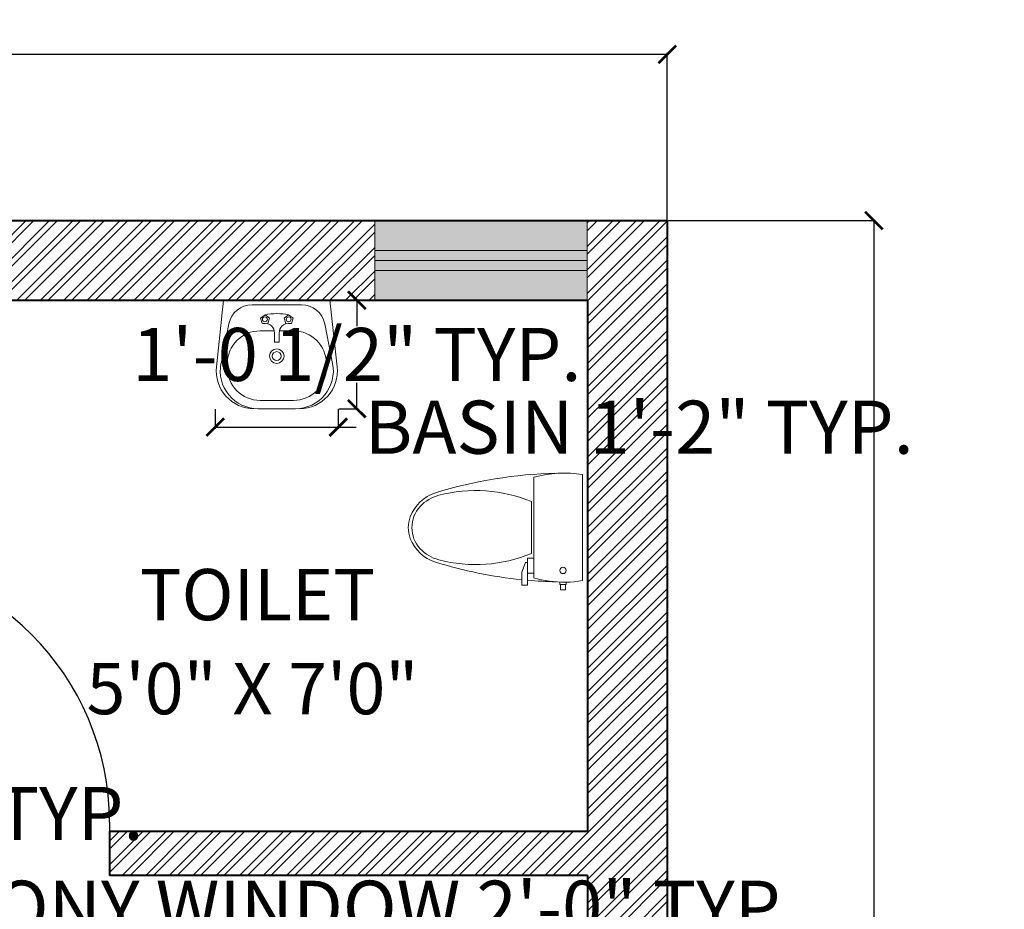
# Model space of a CAD drawing. Units: inches. Extents: x 528 to 2520, y -151 to 1354.
# Tile 27 of 41: x 1350 to 1461, y 1239 to 1340. Entities that reach past the tile are written whole.
import ezdxf

# ---------------------------------------------------------------- set-up
doc = ezdxf.new("R2010")
doc.units = ezdxf.units.IN
doc.header["$MEASUREMENT"] = 0
for name, color, linetype, lineweight in [('A-ANNO-DIMS', 2, 'Continuous', 18), ('A-AREA-IDEN', 7, 'Continuous', 18), ('A-Door', 150, 'Continuous', 25), ('A-FLOR-FIXT', 9, 'Continuous', 18), ('A-WALL-PATT', 6, 'Continuous', 13), ('walls', 7, 'Continuous', 40), ('WINDOWS', 2, 'Continuous', 20)]:
    doc.layers.add(name, color=color, linetype=linetype, lineweight=lineweight)
doc.layers.add('A-GLAZ-PATT', color=152, linetype='Continuous', lineweight=13, true_color=0x2776bb)
doc.styles.get("Standard").update_dxf_attribs({"font": 'arial.ttf'})
doc.dimstyles.get("Standard").update_dxf_attribs({"dimtxt": 6, "dimasz": 2, "dimexe": 0.18, "dimexo": 0.0625, "dimgap": 0.09, "dimtad": 0, "dimtih": 1, "dimtoh": 1, "dimdec": 1, "dimzin": 0, "dimdsep": 46, "dimlunit": 3, "dimtxsty": 'Standard', "dimblk": 'ARCHTICK', "dimcen": 0.09, "dimadec": 0, "dimazin": 0, "dimtfac": 1, "dimtdec": 1, "dimtofl": 0, "dimtmove": 0, "dimatfit": 3, "dimfxl": 1, "dimtolj": 1, "dimtzin": 0, "dimarcsym": 0})

# ---------------------------------------------------------------- blocks, each defined once
blk = doc.blocks.new('toilet-7')
at = {"color": 0, "linetype": 'ByBlock'}
for p, q in [((0.2097, -0.02), (-0.2097, -0.02)), ((0.2151, -0.0677), (0.2097, -0.02)), ((0.2151, -0.1171), (0.2151, -0.0677)), ((-0.2457, -0.0874), (-0.2457, -0.1068)), ((-0.2457, -0.0874), (-0.2257, -0.0874)), ((-0.2457, -0.1068), (-0.2257, -0.1068)), ((-0.2257, -0.0846), (-0.2257, -0.1096)), ((-0.2257, -0.0846), (-0.2157, -0.0846)), ((-0.2257, -0.1096), (-0.2154, -0.1096)), ((0.2099, -0.164), (0.2151, -0.1171)), ((0.1991, -0.2124), (0.2099, -0.164)), ((0.1991, -0.2124), (-0.1991, -0.2124)), ((-0.1803, -0.2374), (-0.1803, -0.2124)), ((-0.1213, -0.2374), (-0.1213, -0.2124)), ((-0.1023, -0.2212), (0.1023, -0.2212)), ((-0.1213, -0.2374), (-0.2278, -0.2374)), ((-0.2278, -0.2374), (-0.2278, -0.2599)), ((-0.1759, -0.2599), (-0.2278, -0.2599)), ((-0.1759, -0.2599), (-0.1379, -0.2451)), ((-0.1379, -0.2451), (-0.1379, -0.2374))]:
    blk.add_line(p, q, dxfattribs=at)
blk.add_circle((-0.1696, -0.0971), 0.0125, dxfattribs=at)
for centre, radius, start, end in [((0.2244, -0.0924), 0.4402, 170.5377, 187.7399), ((1.517, -0.087), 1.7318, 181.2224, 184.9822), ((0.2244, -0.0924), 0.4402, 187.7399, 195.822), ((-1.517, -0.087), 1.7318, 342.7523, 358.7776), ((0.4258, -0.4413), 0.5721, 157.3737, 194.7786), ((-0.4258, -0.4413), 0.5721, 345.2214, 22.6263), ((1.517, -0.087), 1.7318, 185.7323, 197.2477), ((0.0116, -0.5544), 0.1554, 197.2477, 249.5476), ((0.0221, -0.5478), 0.1546, 194.7786, 226.8543), ((-0.0116, -0.5544), 0.1554, 290.4524, 342.7523), ((-0.0221, -0.5478), 0.1546, 313.1457, 345.2214), ((0, -0.5713), 0.1223, 226.8543, 313.1457), ((0, -0.5854), 0.1223, 249.5476, 290.4524)]:
    blk.add_arc(centre, radius, start, end, dxfattribs=at)
blk = doc.blocks.new('_ArchTick')
at = {"color": 0, "linetype": 'ByBlock', "const_width": 0.15}
blk.add_lwpolyline([(-0.5, -0.5), (0.5, 0.5)], dxfattribs=at)
blk = doc.blocks.new('*D26')
at = {"layer": 'A-ANNO-DIMS', "color": 0, "lineweight": -2, "transparency": 16777216}
for p, q in [((1422.95, 1317.1), (1446.41, 1317.1)), ((1446.23, 1317.1), (1446.23, 1069.76)), ((1446.23, 816.1), (1446.23, 1063.45)), ((1422.95, 816.1), (1446.41, 816.1))]:
    blk.add_line(p, q, dxfattribs=at)
at = {"layer": 'Defpoints', "color": 0, "transparency": 16777216}
for p in [(1422.88, 1317.1), (1422.88, 816.1), (1446.23, 816.1)]:
    blk.add_point(p, dxfattribs=at)
at = {"layer": 'A-ANNO-DIMS', "color": 0, "lineweight": -2, "transparency": 16777216, "xscale": 2, "yscale": 2, "zscale": 2}
for p, rotation in [((1446.23, 1317.1), 90), ((1446.23, 816.1), 270)]:
    blk.add_blockref('_ArchTick', p, dxfattribs=dict(at, rotation=rotation))
at = {"layer": 'A-ANNO-DIMS', "color": 0, "transparency": 16777216, "insert": (1446.23, 1066.6), "char_height": 6, "attachment_point": 5}
blk.add_mtext('\\A1;41\'-9.0"', dxfattribs=at)
blk = doc.blocks.new('*D27')
at = {"layer": 'A-ANNO-DIMS', "color": 0, "lineweight": -2, "transparency": 16777216}
for p, q in [((1123.88, 1317.17), (1123.88, 1336.05)), ((1123.88, 1335.87), (1257.11, 1335.87)), ((1422.88, 1335.87), (1289.66, 1335.87)), ((1422.88, 1317.17), (1422.88, 1336.05))]:
    blk.add_line(p, q, dxfattribs=at)
at = {"layer": 'Defpoints', "color": 0, "transparency": 16777216}
for p in [(1422.88, 1335.87), (1123.88, 1317.1), (1422.88, 1317.1)]:
    blk.add_point(p, dxfattribs=at)
at = {"layer": 'A-ANNO-DIMS', "color": 0, "lineweight": -2, "transparency": 16777216, "xscale": 2, "yscale": 2, "zscale": 2, "rotation": 180}
blk.add_blockref('_ArchTick', (1123.88, 1335.87), dxfattribs=at)
at = {"layer": 'A-ANNO-DIMS', "color": 0, "lineweight": -2, "transparency": 16777216, "xscale": 2, "yscale": 2, "zscale": 2}
blk.add_blockref('_ArchTick', (1422.88, 1335.87), dxfattribs=at)
at = {"layer": 'A-ANNO-DIMS', "color": 0, "transparency": 16777216, "insert": (1273.38, 1335.87), "char_height": 6, "attachment_point": 5}
blk.add_mtext('\\A1;24\'-11.0"', dxfattribs=at)
blk = doc.blocks.new('BASIN-WITH-TAP')
for p, q in [((0.84, 12.27), (0.02, 4.73)), ((12.84, 12.27), (0.84, 12.27)), ((12.84, 12.27), (13.66, 4.73)), ((9.64, 11.73), (4.05, 11.73)), ((5, 10.24), (5.51, 10.61)), ((5.2, 9.64), (5, 10.24)), ((5.24, 10.1), (5.2, 10.1)), ((5.51, 10.61), (6.02, 10.24)), ((6.02, 10.24), (5.82, 9.64)), ((8.18, 10.61), (7.67, 10.24)), ((7.67, 10.24), (7.86, 9.64)), ((8.68, 10.24), (8.18, 10.61)), ((8.44, 10.1), (8.49, 10.1)), ((8.49, 9.64), (8.68, 10.24)), ((1.43, 9.58), (0.55, 5.09)), ((5.24, 9.64), (5.51, 9.64)), ((8.49, 9.64), (8.18, 9.64)), ((12.26, 9.58), (13.14, 5.09)), ((4.98, 8.8), (6.58, 8.8)), ((6.58, 8.31), (6.58, 8.58)), ((6.58, 7.51), (6.58, 8.31)), ((8.71, 8.8), (7.11, 8.8)), ((7.11, 8.31), (7.11, 8.58)), ((7.11, 7.51), (7.11, 8.31)), ((6.58, 7.51), (7.11, 7.51)), ((1.24, 4.67), (1.24, 5.07)), ((12.44, 4.67), (12.44, 5.07)), ((4.73, 0), (8.96, 0)), ((6.84, 0.93), (4.98, 0.93)), ((6.84, 0.93), (8.71, 0.93))]:
    blk.add_line(p, q)
for centre, radius in [((5.5, 10.1), 0.277), ((8.19, 10.1), 0.277), ((6.84, 5.94), 0.821), ((6.84, 5.94), 0.507)]:
    blk.add_circle(centre, radius)
for centre, radius, start, end in [((4.05, 9.07), 2.67, 90, 168.8773), ((9.64, 9.07), 2.67, 11.1227, 90), ((6.84, 4.01), 6.73, 78.5788, 101.4212), ((5.51, 8.58), 1.07, 0, 90), ((8.18, 8.58), 1.07, 90, 180), ((4.98, 5.07), 3.73, 90, 180), ((8.71, 5.07), 3.73, 0, 90), ((4.27, 4.27), 4.27, 173.7966, 270), ((4.73, 4.27), 4.27, 168.8773, 270), ((4.98, 4.67), 3.73, 180, 270), ((8.71, 4.67), 3.73, 270, 0), ((8.96, 4.27), 4.27, 270, 11.1227), ((9.42, 4.27), 4.27, 270, 6.2034)]:
    blk.add_arc(centre, radius, start, end)
blk = doc.blocks.new('DOOR-SWING-30')
for p, q in [((0, 6), (0, 0)), ((30, 6), (30, 0))]:
    blk.add_line(p, q)
blk.add_lwpolyline([(0, 6), (0, 36), (1.75, 36), (1.75, 6)], close=True)
blk.add_arc((0, 6), 30, 0, 90)
blk = doc.blocks.new('WINDOW-24x9-PLAN')
for p, q in [((0, 5.63), (24, 5.63)), ((0, 4.5), (24, 4.5)), ((0, 3.37), (24, 3.37))]:
    blk.add_line(p, q)
blk.add_lwpolyline([(0, 9), (24, 9), (24, 0), (0, 0)], close=True)
blk = doc.blocks.new('*D52')
at = {"layer": 'A-ANNO-DIMS', "color": 0, "lineweight": -2, "transparency": 16777216}
for p, q in [((1371.83, 1295.77), (1371.83, 1293.57)), ((1385.73, 1295.77), (1385.73, 1293.57)), ((1371.83, 1293.75), (1385.73, 1293.75)), ((1385.73, 1293.75), (1387.73, 1293.75))]:
    blk.add_line(p, q, dxfattribs=at)
at = {"layer": 'Defpoints', "color": 0, "transparency": 16777216}
for p in [(1371.83, 1295.84), (1385.73, 1295.84), (1385.73, 1293.75)]:
    blk.add_point(p, dxfattribs=at)
at = {"layer": 'A-ANNO-DIMS', "color": 0, "lineweight": -2, "transparency": 16777216, "xscale": 2, "yscale": 2, "zscale": 2, "rotation": 180}
blk.add_blockref('_ArchTick', (1371.83, 1293.75), dxfattribs=at)
at = {"layer": 'A-ANNO-DIMS', "color": 0, "lineweight": -2, "transparency": 16777216, "xscale": 2, "yscale": 2, "zscale": 2}
blk.add_blockref('_ArchTick', (1385.73, 1293.75), dxfattribs=at)
at = {"layer": 'A-ANNO-DIMS', "color": 0, "transparency": 16777216, "insert": (1419.72, 1293.75), "char_height": 6, "attachment_point": 5}
blk.add_mtext('\\A1;BASIN 1\'-2" TYP.', dxfattribs=at)
blk = doc.blocks.new('*D53')
at = {"layer": 'A-ANNO-DIMS', "color": 0, "lineweight": -2, "transparency": 16777216}
for p, q in [((1385.8, 1308.1), (1388, 1308.1)), ((1387.82, 1308.1), (1387.82, 1305.16)), ((1387.82, 1295.84), (1387.82, 1298.78)), ((1385.8, 1295.84), (1388, 1295.84))]:
    blk.add_line(p, q, dxfattribs=at)
at = {"layer": 'Defpoints', "color": 0, "transparency": 16777216}
for p in [(1385.73, 1308.1), (1387.82, 1308.1), (1385.73, 1295.84)]:
    blk.add_point(p, dxfattribs=at)
at = {"layer": 'A-ANNO-DIMS', "color": 0, "lineweight": -2, "transparency": 16777216, "xscale": 2, "yscale": 2, "zscale": 2}
for p, rotation in [((1387.82, 1308.1), 90), ((1387.82, 1295.84), 270)]:
    blk.add_blockref('_ArchTick', p, dxfattribs=dict(at, rotation=rotation))
at = {"layer": 'A-ANNO-DIMS', "color": 0, "transparency": 16777216, "insert": (1387.82, 1301.97), "char_height": 6, "attachment_point": 5}
blk.add_mtext('\\A1;1\'-0 1/2" TYP.', dxfattribs=at)
blk = doc.blocks.new('*D86')
at = {"layer": 'A-ANNO-DIMS', "color": 0, "lineweight": -2, "transparency": 16777216}
for p, q in [((1297.45, 1243.04), (1297.45, 1239.32)), ((1321.45, 1243.04), (1321.45, 1239.32)), ((1297.45, 1239.5), (1321.45, 1239.5)), ((1321.45, 1239.5), (1323.45, 1239.5))]:
    blk.add_line(p, q, dxfattribs=at)
at = {"layer": 'Defpoints', "color": 0, "transparency": 16777216}
for p in [(1297.45, 1243.1), (1321.45, 1243.1), (1321.45, 1239.5)]:
    blk.add_point(p, dxfattribs=at)
at = {"layer": 'A-ANNO-DIMS', "color": 0, "lineweight": -2, "transparency": 16777216, "xscale": 2, "yscale": 2, "zscale": 2, "rotation": 180}
blk.add_blockref('_ArchTick', (1297.45, 1239.5), dxfattribs=at)
at = {"layer": 'A-ANNO-DIMS', "color": 0, "lineweight": -2, "transparency": 16777216, "xscale": 2, "yscale": 2, "zscale": 2}
blk.add_blockref('_ArchTick', (1321.45, 1239.5), dxfattribs=at)
at = {"layer": 'A-ANNO-DIMS', "color": 0, "transparency": 16777216, "insert": (1382.44, 1239.5), "char_height": 6, "attachment_point": 5}
blk.add_mtext('\\A1;BALCONY WINDOW 2\'-0" TYP.', dxfattribs=at)
blk = doc.blocks.new('*D87')
at = {"layer": 'A-ANNO-DIMS', "color": 0, "lineweight": -2, "transparency": 16777216}
for p, q in [((1325.05, 1248.1), (1325.05, 1250.1)), ((1325.05, 1250.1), (1327.05, 1250.1)), ((1321.51, 1248.1), (1325.23, 1248.1)), ((1325.05, 1243.1), (1325.05, 1248.1)), ((1321.51, 1243.1), (1325.23, 1243.1))]:
    blk.add_line(p, q, dxfattribs=at)
at = {"layer": 'Defpoints', "color": 0, "transparency": 16777216}
for p in [(1321.45, 1248.1), (1325.05, 1248.1), (1321.45, 1243.1)]:
    blk.add_point(p, dxfattribs=at)
at = {"layer": 'A-ANNO-DIMS', "color": 0, "lineweight": -2, "transparency": 16777216, "xscale": 2, "yscale": 2, "zscale": 2}
for p, rotation in [((1325.05, 1248.1), 90), ((1325.05, 1243.1), 270)]:
    blk.add_blockref('_ArchTick', p, dxfattribs=dict(at, rotation=rotation))
at = {"layer": 'A-ANNO-DIMS', "color": 0, "transparency": 16777216, "insert": (1345.43, 1250.1), "char_height": 6, "attachment_point": 5}
blk.add_mtext('\\A1;0\'-5" TYP.', dxfattribs=at)

msp = doc.modelspace()

# ---------------------------------------------------------------- hatches: boundary and pattern name
at = {"layer": 'A-GLAZ-PATT'}
h = msp.add_hatch(color=256, dxfattribs=at)
h.dxf.hatch_style = 1
h.paths.add_polyline_path([(1413.84, 1313.73), (1389.84, 1313.73), (1389.84, 1312.6), (1413.84, 1312.6)])
h.paths.add_polyline_path([(1413.84, 1312.6), (1389.84, 1312.6), (1389.84, 1311.47), (1413.84, 1311.47)])
h.paths.add_polyline_path([(1413.84, 1317.1), (1389.84, 1317.1), (1389.84, 1313.73), (1413.84, 1313.73)])
h.paths.add_polyline_path([(1413.84, 1311.47), (1389.84, 1311.47), (1389.84, 1308.1), (1413.84, 1308.1)])
at = {"layer": 'A-WALL-PATT'}
h = msp.add_hatch(dxfattribs=at)
h.set_pattern_fill('ANSI32', color=256, scale=5)
h.set_pattern_definition([(45, (537.1868, 0), (-1.3258252, 1.3258252), []), (45, (538.0707, 0), (-1.3258252, 1.3258252), [])])
h.paths.add_polyline_path([(1132.88, 1163.86), (1123.88, 1163.86), (1123.88, 969.1), (1135.43, 969.1), (1140.43, 969.1), (1140.43, 974.1), (1132.88, 974.1), (1132.88, 1082.1), (1228.88, 1082.1), (1228.88, 1087.1), (1228.88, 1106.1), (1234.88, 1106.1), (1234.88, 1111.1), (1223.88, 1111.1), (1223.88, 1087.1), (1132.88, 1087.1)])
h.paths.add_polyline_path([(1225.89, 974.1), (1188.43, 974.1), (1188.43, 969.1), (1225.89, 969.1)])
h.paths.add_polyline_path([(1422.88, 1171.37), (1413.88, 1171.37), (1413.88, 1111.1), (1323.88, 1111.1), (1323.88, 1106.1), (1413.88, 1106.1), (1413.88, 974.1), (1323.88, 974.1), (1323.88, 969.1), (1413.88, 969.1), (1413.88, 825.1), (1371.88, 825.1), (1371.88, 816.1), (1422.88, 816.1)])
h.paths.add_polyline_path([(1422.88, 1317.1), (1413.84, 1317.1), (1413.84, 1308.1), (1413.88, 1308.1), (1413.88, 1248.1), (1359.88, 1248.1), (1359.88, 1243.1), (1413.88, 1243.1), (1413.88, 1219.37), (1422.88, 1219.37)])
h.paths.add_polyline_path([(1389.84, 1317.1), (1324.88, 1317.1), (1324.88, 1248.1), (1321.45, 1248.1), (1321.45, 1243.1), (1329.88, 1243.1), (1329.88, 1249.1), (1329.88, 1308.1), (1389.84, 1308.1)])
h.paths.add_polyline_path([(1221.88, 1317.1), (1156.88, 1317.1), (1156.88, 1308.1), (1216.88, 1308.1), (1216.88, 1248.1), (1216.88, 1243.1), (1221.88, 1243.1), (1221.88, 1248.25)])
h.paths.add_polyline_path([(1132.88, 1308.1), (1132.88, 1317.1), (1123.88, 1317.1), (1123.88, 1211.86), (1132.88, 1211.86), (1132.88, 1243.1), (1186.88, 1243.1), (1186.88, 1248.1), (1132.88, 1248.1)])
h.paths.add_polyline_path([(1281.88, 969.1), (1281.88, 974.1), (1261.89, 974.1), (1261.89, 969.1), (1276.88, 969.1), (1276.88, 874.29), (1281.88, 874.29)])
h.paths.add_polyline_path([(1276.88, 969.1), (1264.88, 969.1), (1264.88, 965.12), (1267.92, 965.12), (1267.92, 961.68), (1271.62, 961.68), (1271.62, 957.24), (1276.88, 957.24)], flags=17)
h.paths.add_polyline_path([(1323.88, 825.1), (1281.88, 825.1), (1281.88, 832.29), (1276.88, 832.29), (1276.88, 816.1), (1323.88, 816.1)])

# ---------------------------------------------------------------- linework, layer by layer
at = {"layer": 'walls'}
for p, q in [((1324.88, 1317.1), (1422.88, 1317.1)), ((1422.88, 1317.1), (1422.88, 816.1)), ((1329.88, 1308.1), (1413.88, 1308.1)), ((1413.88, 1308.1), (1413.88, 1248.1)), ((1359.88, 1248.1), (1413.88, 1248.1)), ((1359.88, 1248.1), (1359.88, 1243.1)), ((1413.88, 1243.1), (1359.88, 1243.1)), ((1413.88, 1243.1), (1413.88, 1111.1))]:
    msp.add_line(p, q, dxfattribs=at)

# ---------------------------------------------------------------- block references
at = {"layer": 'A-Door'}
msp.add_blockref('DOOR-SWING-30', (1329.88, 1243.1), dxfattribs=at)
at = {"layer": 'A-FLOR-FIXT'}
msp.add_blockref('BASIN-WITH-TAP', (1371.94, 1295.84), dxfattribs=at)
at = {"layer": 'A-FLOR-FIXT', "xscale": -28.60654769571749, "yscale": 28.60654769571749, "zscale": 28.60654769571749, "rotation": 270}
msp.add_blockref('toilet-7', (1413.88, 1282.41), dxfattribs=at)
at = {"layer": 'WINDOWS'}
msp.add_blockref('WINDOW-24x9-PLAN', (1389.84, 1308.1), dxfattribs=at)

# ---------------------------------------------------------------- texts
at = {"layer": 'A-AREA-IDEN'}
for s, height, p in [('TOILET', 5.793, (1363.3, 1271.93)), ('5\'0" X 7\'0"', 5.7926, (1357.29, 1261.31))]:
    msp.add_text(s, height=height, dxfattribs=at).set_placement(p)

# ---------------------------------------------------------------- dimensions: what is measured, and where the dimension line sits
at = {"layer": 'A-ANNO-DIMS'}
dim = msp.add_linear_dim(base=(1422.88, 1335.87), p1=(1123.88, 1317.1), p2=(1422.88, 1317.1), dimstyle='Standard', override={"dimclrd": 0, "dimclre": 0, "dimclrt": 0}, dxfattribs=at)
dim.commit()
dim.dimension.update_dxf_attribs({"geometry": '*D27', "text_midpoint": (1273.38, 1335.87)})
dim = msp.add_linear_dim(base=(1446.23, 816.1), p1=(1422.88, 1317.1), p2=(1422.88, 816.1), angle=90, dimstyle='Standard', override={"dimclrd": 0, "dimclre": 0, "dimclrt": 0}, dxfattribs=at)
dim.commit()
dim.dimension.update_dxf_attribs({"geometry": '*D26', "text_midpoint": (1446.23, 1066.6)})
for base, p1, p2, picture, middle in [((1387.82, 1308.1), (1385.73, 1295.84), (1385.73, 1308.1), '*D53', (1387.82, 1301.97)), ((1325.05, 1248.1), (1321.45, 1243.1), (1321.45, 1248.1), '*D87', (1345.43, 1250.1))]:
    dim = msp.add_linear_dim(base=base, p1=p1, p2=p2, angle=90, text='<> TYP.', dimstyle='Standard', override={"dimdec": 1, "dimlfac": 1, "dimrnd": 0, "dimzin": 1, "dimdsep": 46, "dimlunit": 4, "dimfrac": 2}, dxfattribs=at)
    dim.commit()
    dim.dimension.update_dxf_attribs({"geometry": picture, "text_midpoint": middle})
for base, p1, p2, text, picture, middle in [((1385.73, 1293.75), (1371.83, 1295.84), (1385.73, 1295.84), 'BASIN <> TYP.', '*D52', (1419.72, 1293.75)), ((1321.45, 1239.5), (1297.45, 1243.1), (1321.45, 1243.1), 'BALCONY WINDOW <> TYP.', '*D86', (1382.44, 1239.5))]:
    dim = msp.add_linear_dim(base=base, p1=p1, p2=p2, text=text, dimstyle='Standard', override={"dimdec": 1, "dimlfac": 1, "dimrnd": 0, "dimzin": 1, "dimdsep": 46, "dimlunit": 4, "dimfrac": 2}, dxfattribs=at)
    dim.commit()
    dim.dimension.update_dxf_attribs({"geometry": picture, "text_midpoint": middle})

doc.saveas('drawing.dxf')
